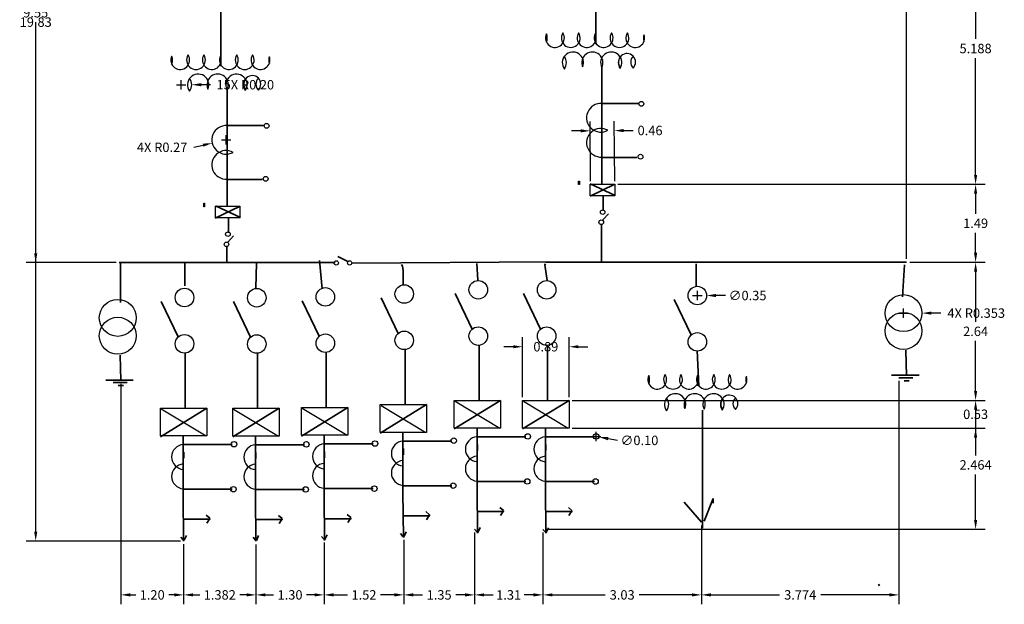
# Model space of a CAD drawing. Units: millimetres. Extents: x -4 to 31.8, y -11 to 11.2.
# Tile 1 of 2: x 13 to 31.8, y -11 to 0.1. Entities that reach past the tile are written whole.
import ezdxf

# ---------------------------------------------------------------- set-up
doc = ezdxf.new("R2010")
doc.units = ezdxf.units.MM
doc.header["$MEASUREMENT"] = 0
for name, color, linetype, lineweight in [('A-ANNO-DIMS', 2, 'Continuous', 18), ('E-ONEL-WIRE', 7, 'Continuous', 35), ('E-POWR-EQPM', 4, 'Continuous', 25)]:
    doc.layers.add(name, color=color, linetype=linetype, lineweight=lineweight)
doc.styles.get("Standard").update_dxf_attribs({"font": 'arial.ttf'})
doc.dimstyles.get("Standard").update_dxf_attribs({"dimtxt": 0.18, "dimasz": 0.18, "dimexe": 0.18, "dimexo": 0.0625, "dimgap": 0.09, "dimtad": 0, "dimtih": 1, "dimtoh": 1, "dimdec": 4, "dimzin": 0, "dimdsep": 46, "dimtxsty": 'Standard', "dimcen": 0.09, "dimadec": 0, "dimazin": 0, "dimtfac": 1, "dimtdec": 4, "dimtofl": 0, "dimtmove": 0, "dimatfit": 3, "dimfxl": 1, "dimtolj": 1, "dimtzin": 0, "dimarcsym": 0})

# ---------------------------------------------------------------- blocks, each defined once
blk = doc.blocks.new('XFMR-POWER')
for centre, radius, start, end in [((16.061, -0.651), 0.18, 154.6992, 32.9126), ((16.363, -0.651), 0.18, 147.0874, 32.9126), ((16.666, -0.651), 0.18, 147.0874, 25.3007), ((16.992, -0.651), 0.18, 154.6993, 32.9127), ((17.294, -0.651), 0.18, 147.0873, 32.9126), ((17.596, -0.651), 0.18, 147.0874, 20.5503), ((15.735, -0.651), 0.18, 334.6992, 25.3008), ((17.934, -0.651), 0.18, 159.4497, 200.5503), ((16.404, -1.122), 0.203, 336.2266, 216.7978), ((16.776, -1.122), 0.203, 332.4427, 203.7734), ((17.137, -1.122), 0.203, 326.0323, 207.5573), ((16.078, -1.122), 0.203, 323.2022, 36.7978), ((17.474, -1.122), 0.203, 146.0323, 213.9677), ((17.439, -1.11), 0.163, 315.5847, 221.0573), ((17.672, -1.11), 0.163, 135.5847, 224.4153)]:
    blk.add_arc(centre, radius, start, end)
blk = doc.blocks.new('CB-BREAKER')
blk.add_line((15.7, -7.316), (16.556, -7.832))
blk.add_lwpolyline([(15.685, -7.301), (16.571, -7.301), (16.571, -7.832), (15.685, -7.832)], close=True)
blk = doc.blocks.new('XFMR-AUX-LARGE')
for centre in [(14.868, -5.577), (14.868, -5.918)]:
    blk.add_circle(centre, 0.353)
blk = doc.blocks.new('*D7')
at = {"layer": 'A-ANNO-DIMS', "color": 0, "lineweight": -2, "transparency": 16777216}
for p, q in [((14.324, 5.091), (14.324, 11.195)), ((29.944, -4.451), (29.944, 11.195)), ((14.504, 11.015), (21.75, 11.015)), ((29.764, 11.015), (22.518, 11.015))]:
    blk.add_line(p, q, dxfattribs=at)
at = {"layer": 'A-ANNO-DIMS', "color": 0, "transparency": 16777216}
for points in [[(14.504, 11.045), (14.504, 10.985), (14.324, 11.015)], [(29.764, 11.045), (29.764, 10.985), (29.944, 11.015)]]:
    blk.add_solid(points, dxfattribs=at)
at = {"layer": 'Defpoints', "color": 0, "transparency": 16777216}
for p in [(29.944, 11.015), (14.324, 5.028), (29.944, -4.514)]:
    blk.add_point(p, dxfattribs=at)
at = {"layer": 'A-ANNO-DIMS', "color": 0, "transparency": 16777216, "insert": (22.134, 11.015), "char_height": 0.18, "attachment_point": 5}
blk.add_mtext('\\A1;15.62', dxfattribs=at)
blk = doc.blocks.new('*D13')
at = {"layer": 'A-ANNO-DIMS', "color": 0, "lineweight": -2, "transparency": 16777216}
for p, q in [((19.924, 9.99), (13.119, 9.99)), ((13.299, 9.81), (13.299, 0.256)), ((13.299, -9.661), (13.299, -0.108)), ((16.065, -9.841), (13.119, -9.841))]:
    blk.add_line(p, q, dxfattribs=at)
at = {"layer": 'A-ANNO-DIMS', "color": 0, "transparency": 16777216}
for points in [[(13.269, 9.81), (13.329, 9.81), (13.299, 9.99)], [(13.269, -9.661), (13.329, -9.661), (13.299, -9.841)]]:
    blk.add_solid(points, dxfattribs=at)
at = {"layer": 'Defpoints', "color": 0, "transparency": 16777216}
for p in [(13.299, 9.99), (19.987, 9.99), (16.127, -9.841)]:
    blk.add_point(p, dxfattribs=at)
at = {"layer": 'A-ANNO-DIMS', "color": 0, "transparency": 16777216, "insert": (13.299, 0.074), "char_height": 0.18, "attachment_point": 5}
blk.add_mtext('\\A1;19.83', dxfattribs=at)
blk = doc.blocks.new('*D14')
at = {"layer": 'A-ANNO-DIMS', "color": 0, "lineweight": -2, "transparency": 16777216}
for p, q in [((14.262, 5.028), (13.119, 5.028)), ((13.299, 4.848), (13.299, 0.435)), ((13.299, -4.342), (13.299, 0.071)), ((14.834, -4.522), (13.119, -4.522))]:
    blk.add_line(p, q, dxfattribs=at)
at = {"layer": 'A-ANNO-DIMS', "color": 0, "transparency": 16777216}
for points in [[(13.269, 4.848), (13.329, 4.848), (13.299, 5.028)], [(13.269, -4.342), (13.329, -4.342), (13.299, -4.522)]]:
    blk.add_solid(points, dxfattribs=at)
at = {"layer": 'Defpoints', "color": 0, "transparency": 16777216}
for p in [(13.299, 5.028), (14.324, 5.028), (14.897, -4.522)]:
    blk.add_point(p, dxfattribs=at)
at = {"layer": 'A-ANNO-DIMS', "color": 0, "transparency": 16777216, "insert": (13.299, 0.253), "char_height": 0.18, "attachment_point": 5}
blk.add_mtext('\\A1;9.55', dxfattribs=at)
blk = doc.blocks.new('*D18')
at = {"layer": 'A-ANNO-DIMS', "color": 0, "lineweight": -2, "transparency": 16777216}
for p, q in [((24.519, 2.164), (31.446, 2.164)), ((31.266, 1.984), (31.266, -0.248)), ((31.266, -2.844), (31.266, -0.612)), ((24.43, -3.024), (31.446, -3.024))]:
    blk.add_line(p, q, dxfattribs=at)
at = {"layer": 'A-ANNO-DIMS', "color": 0, "transparency": 16777216}
for points in [[(31.236, 1.984), (31.296, 1.984), (31.266, 2.164)], [(31.236, -2.844), (31.296, -2.844), (31.266, -3.024)]]:
    blk.add_solid(points, dxfattribs=at)
at = {"layer": 'Defpoints', "color": 0, "transparency": 16777216}
for p in [(24.456, 2.164), (31.266, 2.164), (24.367, -3.024)]:
    blk.add_point(p, dxfattribs=at)
at = {"layer": 'A-ANNO-DIMS', "color": 0, "transparency": 16777216, "insert": (31.266, -0.43), "char_height": 0.18, "attachment_point": 5}
blk.add_mtext('\\A1;5.188', dxfattribs=at)
blk = doc.blocks.new('*D19')
at = {"layer": 'A-ANNO-DIMS', "color": 0, "lineweight": -2, "transparency": 16777216}
for p, q in [((24.43, -3.024), (31.446, -3.024)), ((31.266, -3.204), (31.266, -3.587)), ((31.266, -4.334), (31.266, -3.951)), ((30.006, -4.514), (31.446, -4.514))]:
    blk.add_line(p, q, dxfattribs=at)
at = {"layer": 'A-ANNO-DIMS', "color": 0, "transparency": 16777216}
for points in [[(31.236, -3.204), (31.296, -3.204), (31.266, -3.024)], [(31.236, -4.334), (31.296, -4.334), (31.266, -4.514)]]:
    blk.add_solid(points, dxfattribs=at)
at = {"layer": 'Defpoints', "color": 0, "transparency": 16777216}
for p in [(24.367, -3.024), (31.266, -3.024), (29.944, -4.514)]:
    blk.add_point(p, dxfattribs=at)
at = {"layer": 'A-ANNO-DIMS', "color": 0, "transparency": 16777216, "insert": (31.266, -3.769), "char_height": 0.18, "attachment_point": 5}
blk.add_mtext('\\A1;1.49', dxfattribs=at)
blk = doc.blocks.new('*D20')
at = {"layer": 'A-ANNO-DIMS', "color": 0, "lineweight": -2, "transparency": 16777216}
for p, q in [((30.006, -4.514), (31.446, -4.514)), ((31.266, -4.694), (31.266, -5.652)), ((31.266, -6.974), (31.266, -6.016)), ((23.556, -7.154), (31.446, -7.154))]:
    blk.add_line(p, q, dxfattribs=at)
at = {"layer": 'A-ANNO-DIMS', "color": 0, "transparency": 16777216}
for points in [[(31.236, -4.694), (31.296, -4.694), (31.266, -4.514)], [(31.236, -6.974), (31.296, -6.974), (31.266, -7.154)]]:
    blk.add_solid(points, dxfattribs=at)
at = {"layer": 'Defpoints', "color": 0, "transparency": 16777216}
for p in [(29.944, -4.514), (31.266, -4.514), (23.494, -7.154)]:
    blk.add_point(p, dxfattribs=at)
at = {"layer": 'A-ANNO-DIMS', "color": 0, "transparency": 16777216, "insert": (31.266, -5.834), "char_height": 0.18, "attachment_point": 5}
blk.add_mtext('\\A1;2.64', dxfattribs=at)
blk = doc.blocks.new('*D21')
at = {"layer": 'A-ANNO-DIMS', "color": 0, "lineweight": -2, "transparency": 16777216}
for p, q in [((23.556, -7.154), (31.446, -7.154)), ((31.266, -7.334), (31.266, -8.204)), ((31.266, -9.437), (31.266, -8.567)), ((23.056, -9.617), (31.446, -9.617))]:
    blk.add_line(p, q, dxfattribs=at)
at = {"layer": 'A-ANNO-DIMS', "color": 0, "transparency": 16777216}
for points in [[(31.236, -7.334), (31.296, -7.334), (31.266, -7.154)], [(31.236, -9.437), (31.296, -9.437), (31.266, -9.617)]]:
    blk.add_solid(points, dxfattribs=at)
at = {"layer": 'Defpoints', "color": 0, "transparency": 16777216}
for p in [(23.494, -7.154), (31.266, -7.154), (22.994, -9.617)]:
    blk.add_point(p, dxfattribs=at)
at = {"layer": 'A-ANNO-DIMS', "color": 0, "transparency": 16777216, "insert": (31.266, -8.386), "char_height": 0.18, "attachment_point": 5}
blk.add_mtext('\\A1;2.464', dxfattribs=at)
blk = doc.blocks.new('*D22')
at = {"layer": 'A-ANNO-DIMS', "color": 0, "lineweight": -2, "transparency": 16777216}
for p, q in [((31.266, -6.974), (31.266, -6.794)), ((23.556, -7.154), (31.446, -7.154)), ((23.556, -7.685), (31.446, -7.685)), ((31.266, -7.865), (31.266, -8.045))]:
    blk.add_line(p, q, dxfattribs=at)
at = {"layer": 'A-ANNO-DIMS', "color": 0, "transparency": 16777216}
for points in [[(31.236, -6.974), (31.296, -6.974), (31.266, -7.154)], [(31.236, -7.865), (31.296, -7.865), (31.266, -7.685)]]:
    blk.add_solid(points, dxfattribs=at)
at = {"layer": 'Defpoints', "color": 0, "transparency": 16777216}
for p in [(23.494, -7.154), (23.494, -7.685), (31.266, -7.685)]:
    blk.add_point(p, dxfattribs=at)
at = {"layer": 'A-ANNO-DIMS', "color": 0, "transparency": 16777216, "insert": (31.266, -7.419), "char_height": 0.18, "attachment_point": 5}
blk.add_mtext('\\A1;0.53', dxfattribs=at)
blk = doc.blocks.new('*D23')
at = {"layer": 'A-ANNO-DIMS', "color": 0, "lineweight": -2, "transparency": 16777216}
for p, q in [((14.925612, -6.837922), (14.925612, -11.049806)), ((16.127036, -9.903339), (16.127036, -11.049806)), ((15.105612, -10.869806), (15.211324, -10.869806)), ((15.947036, -10.869806), (15.841324, -10.869806))]:
    blk.add_line(p, q, dxfattribs=at)
at = {"layer": 'A-ANNO-DIMS', "color": 0, "transparency": 16777216}
for points in [[(15.105612, -10.839806), (15.105612, -10.899806), (14.925612, -10.869806)], [(15.947036, -10.839806), (15.947036, -10.899806), (16.127036, -10.869806)]]:
    blk.add_solid(points, dxfattribs=at)
at = {"layer": 'Defpoints', "color": 0, "transparency": 16777216}
for p in [(14.925612, -6.775422), (16.127036, -9.840839), (16.127036, -10.869806)]:
    blk.add_point(p, dxfattribs=at)
at = {"layer": 'A-ANNO-DIMS', "color": 0, "transparency": 16777216, "insert": (15.526324, -10.869806), "char_height": 0.18, "attachment_point": 5}
blk.add_mtext('\\A1;1.20', dxfattribs=at)
blk = doc.blocks.new('*D24')
at = {"layer": 'A-ANNO-DIMS', "color": 0, "lineweight": -2, "transparency": 16777216}
for p, q in [((16.127, -9.903), (16.127, -11.05)), ((17.509, -9.907), (17.509, -11.05)), ((16.307, -10.87), (16.434, -10.87)), ((17.329, -10.87), (17.202, -10.87))]:
    blk.add_line(p, q, dxfattribs=at)
at = {"layer": 'A-ANNO-DIMS', "color": 0, "transparency": 16777216}
for points in [[(16.307, -10.84), (16.307, -10.9), (16.127, -10.87)], [(17.329, -10.84), (17.329, -10.9), (17.509, -10.87)]]:
    blk.add_solid(points, dxfattribs=at)
at = {"layer": 'Defpoints', "color": 0, "transparency": 16777216}
for p in [(16.127, -9.841), (17.509, -9.845), (17.509, -10.87)]:
    blk.add_point(p, dxfattribs=at)
at = {"layer": 'A-ANNO-DIMS', "color": 0, "transparency": 16777216, "insert": (16.818, -10.87), "char_height": 0.18, "attachment_point": 5}
blk.add_mtext('\\A1;1.382', dxfattribs=at)
blk = doc.blocks.new('*D25')
at = {"layer": 'A-ANNO-DIMS', "color": 0, "lineweight": -2, "transparency": 16777216}
for p, q in [((17.509, -9.907), (17.509, -11.05)), ((18.813, -9.872), (18.813, -11.05)), ((17.689, -10.87), (17.846, -10.87)), ((18.633, -10.87), (18.476, -10.87))]:
    blk.add_line(p, q, dxfattribs=at)
at = {"layer": 'A-ANNO-DIMS', "color": 0, "transparency": 16777216}
for points in [[(17.689, -10.84), (17.689, -10.9), (17.509, -10.87)], [(18.633, -10.84), (18.633, -10.9), (18.813, -10.87)]]:
    blk.add_solid(points, dxfattribs=at)
at = {"layer": 'Defpoints', "color": 0, "transparency": 16777216}
for p in [(17.509, -9.845), (18.813, -9.809), (18.813, -10.87)]:
    blk.add_point(p, dxfattribs=at)
at = {"layer": 'A-ANNO-DIMS', "color": 0, "transparency": 16777216, "insert": (18.161, -10.87), "char_height": 0.18, "attachment_point": 5}
blk.add_mtext('\\A1;1.30', dxfattribs=at)
blk = doc.blocks.new('*D26')
at = {"layer": 'A-ANNO-DIMS', "color": 0, "lineweight": -2, "transparency": 16777216}
for p, q in [((18.813, -9.872), (18.813, -11.05)), ((20.336, -9.821), (20.336, -11.05)), ((18.993, -10.87), (19.26, -10.87)), ((20.156, -10.87), (19.889, -10.87))]:
    blk.add_line(p, q, dxfattribs=at)
at = {"layer": 'A-ANNO-DIMS', "color": 0, "transparency": 16777216}
for points in [[(18.993, -10.84), (18.993, -10.9), (18.813, -10.87)], [(20.156, -10.84), (20.156, -10.9), (20.336, -10.87)]]:
    blk.add_solid(points, dxfattribs=at)
at = {"layer": 'Defpoints', "color": 0, "transparency": 16777216}
for p in [(20.336, -9.758), (18.813, -9.809), (20.336, -10.87)]:
    blk.add_point(p, dxfattribs=at)
at = {"layer": 'A-ANNO-DIMS', "color": 0, "transparency": 16777216, "insert": (19.574, -10.87), "char_height": 0.18, "attachment_point": 5}
blk.add_mtext('\\A1;1.52', dxfattribs=at)
blk = doc.blocks.new('*D27')
at = {"layer": 'A-ANNO-DIMS', "color": 0, "lineweight": -2, "transparency": 16777216}
for p, q in [((21.687, -9.679), (21.687, -11.05)), ((20.336, -9.821), (20.336, -11.05)), ((20.516, -10.87), (20.695, -10.87)), ((21.507, -10.87), (21.327, -10.87))]:
    blk.add_line(p, q, dxfattribs=at)
at = {"layer": 'A-ANNO-DIMS', "color": 0, "transparency": 16777216}
for points in [[(20.516, -10.84), (20.516, -10.9), (20.336, -10.87)], [(21.507, -10.84), (21.507, -10.9), (21.687, -10.87)]]:
    blk.add_solid(points, dxfattribs=at)
at = {"layer": 'Defpoints', "color": 0, "transparency": 16777216}
for p in [(20.336, -9.758), (21.687, -9.617), (21.687, -10.87)]:
    blk.add_point(p, dxfattribs=at)
at = {"layer": 'A-ANNO-DIMS', "color": 0, "transparency": 16777216, "insert": (21.011, -10.87), "char_height": 0.18, "attachment_point": 5}
blk.add_mtext('\\A1;1.35', dxfattribs=at)
blk = doc.blocks.new('*D28')
at = {"layer": 'A-ANNO-DIMS', "color": 0, "lineweight": -2, "transparency": 16777216}
for p, q in [((21.687, -9.679), (21.687, -11.05)), ((22.994, -9.68), (22.994, -11.05)), ((21.867, -10.87), (22.042, -10.87)), ((22.814, -10.87), (22.638, -10.87))]:
    blk.add_line(p, q, dxfattribs=at)
at = {"layer": 'A-ANNO-DIMS', "color": 0, "transparency": 16777216}
for points in [[(21.867, -10.84), (21.867, -10.9), (21.687, -10.87)], [(22.814, -10.84), (22.814, -10.9), (22.994, -10.87)]]:
    blk.add_solid(points, dxfattribs=at)
at = {"layer": 'Defpoints', "color": 0, "transparency": 16777216}
for p in [(21.687, -9.617), (22.994, -9.617), (22.994, -10.87)]:
    blk.add_point(p, dxfattribs=at)
at = {"layer": 'A-ANNO-DIMS', "color": 0, "transparency": 16777216, "insert": (22.34, -10.87), "char_height": 0.18, "attachment_point": 5}
blk.add_mtext('\\A1;1.31', dxfattribs=at)
blk = doc.blocks.new('*D29')
at = {"layer": 'A-ANNO-DIMS', "color": 0, "lineweight": -2, "transparency": 16777216}
for p, q in [((26.026, -9.543), (26.026, -11.05)), ((22.994, -9.68), (22.994, -11.05)), ((23.174, -10.87), (24.186, -10.87)), ((25.846, -10.87), (24.833, -10.87))]:
    blk.add_line(p, q, dxfattribs=at)
at = {"layer": 'A-ANNO-DIMS', "color": 0, "transparency": 16777216}
for points in [[(23.174, -10.84), (23.174, -10.9), (22.994, -10.87)], [(25.846, -10.84), (25.846, -10.9), (26.026, -10.87)]]:
    blk.add_solid(points, dxfattribs=at)
at = {"layer": 'Defpoints', "color": 0, "transparency": 16777216}
for p in [(26.026, -9.48), (22.994, -9.617), (26.026, -10.87)]:
    blk.add_point(p, dxfattribs=at)
at = {"layer": 'A-ANNO-DIMS', "color": 0, "transparency": 16777216, "insert": (24.51, -10.87), "char_height": 0.18, "attachment_point": 5}
blk.add_mtext('\\A1;3.03', dxfattribs=at)
blk = doc.blocks.new('*D30')
at = {"layer": 'A-ANNO-DIMS', "color": 0, "lineweight": -2, "transparency": 16777216}
for p, q in [((29.8, -6.783), (29.8, -11.05)), ((26.026, -9.543), (26.026, -11.05)), ((26.206, -10.87), (27.52, -10.87)), ((29.62, -10.87), (28.306, -10.87))]:
    blk.add_line(p, q, dxfattribs=at)
at = {"layer": 'A-ANNO-DIMS', "color": 0, "transparency": 16777216}
for points in [[(26.206, -10.84), (26.206, -10.9), (26.026, -10.87)], [(29.62, -10.84), (29.62, -10.9), (29.8, -10.87)]]:
    blk.add_solid(points, dxfattribs=at)
at = {"layer": 'Defpoints', "color": 0, "transparency": 16777216}
for p in [(29.8, -6.72), (26.026, -9.48), (29.8, -10.87)]:
    blk.add_point(p, dxfattribs=at)
at = {"layer": 'A-ANNO-DIMS', "color": 0, "transparency": 16777216, "insert": (27.913, -10.87), "char_height": 0.18, "attachment_point": 5}
blk.add_mtext('\\A1;3.774', dxfattribs=at)
blk = doc.blocks.new('*D31')
at = {"layer": 'A-ANNO-DIMS', "color": 0, "lineweight": -2, "transparency": 16777216}
for p, q in [((22.607382, -7.091185), (22.607382, -5.948685)), ((23.4935, -7.091185), (23.4935, -5.948685)), ((22.427382, -6.128685), (22.247382, -6.128685)), ((23.6735, -6.128685), (23.8535, -6.128685))]:
    blk.add_line(p, q, dxfattribs=at)
at = {"layer": 'A-ANNO-DIMS', "color": 0, "transparency": 16777216}
for points in [[(22.427382, -6.098685), (22.427382, -6.158685), (22.607382, -6.128685)], [(23.6735, -6.098685), (23.6735, -6.158685), (23.4935, -6.128685)]]:
    blk.add_solid(points, dxfattribs=at)
at = {"layer": 'Defpoints', "color": 0, "transparency": 16777216}
for p in [(23.4935, -6.128685), (22.607382, -7.153685), (23.4935, -7.153685)]:
    blk.add_point(p, dxfattribs=at)
at = {"layer": 'A-ANNO-DIMS', "color": 0, "transparency": 16777216, "insert": (23.050441, -6.128685), "char_height": 0.18, "attachment_point": 5}
blk.add_mtext('\\A1;0.89', dxfattribs=at)
blk = doc.blocks.new('*D33')
at = {"layer": 'A-ANNO-DIMS', "color": 0, "lineweight": -2, "transparency": 16777216}
for p, q in [((23.907, -2.965), (23.898, -1.823)), ((24.367, -2.962), (24.358, -1.819)), ((23.719, -2.004), (23.539, -2.006)), ((24.539, -1.998), (24.719, -1.996))]:
    blk.add_line(p, q, dxfattribs=at)
at = {"layer": 'A-ANNO-DIMS', "color": 0, "transparency": 16777216}
for points in [[(23.719, -1.974), (23.719, -2.034), (23.899, -2.003)], [(24.539, -1.968), (24.539, -2.028), (24.359, -1.999)]]:
    blk.add_solid(points, dxfattribs=at)
at = {"layer": 'Defpoints', "color": 0, "transparency": 16777216}
for p in [(24.359, -1.999), (23.907, -3.028), (24.367, -3.024)]:
    blk.add_point(p, dxfattribs=at)
at = {"layer": 'A-ANNO-DIMS', "color": 0, "transparency": 16777216, "insert": (25.043, -1.996), "char_height": 0.18, "attachment_point": 5}
blk.add_mtext('\\A1;0.46', dxfattribs=at)
blk = doc.blocks.new('*D34')
at = {"layer": 'A-ANNO-DIMS', "color": 0, "lineweight": -2, "transparency": 16777216}
for p, q in [((29.888, -5.576), (29.888, -5.396)), ((29.798, -5.486), (29.978, -5.486)), ((30.601, -5.486), (30.421, -5.486))]:
    blk.add_line(p, q, dxfattribs=at)
at = {"layer": 'A-ANNO-DIMS', "color": 0, "transparency": 16777216}
blk.add_solid([(30.421, -5.456), (30.421, -5.516), (30.241, -5.486)], dxfattribs=at)
at = {"layer": 'Defpoints', "color": 0, "transparency": 16777216}
for p in [(29.888, -5.486), (30.241, -5.486)]:
    blk.add_point(p, dxfattribs=at)
at = {"layer": 'A-ANNO-DIMS', "color": 0, "transparency": 16777216, "insert": (31.278, -5.486), "char_height": 0.18, "attachment_point": 5}
blk.add_mtext('\\A1;4X R0.353', dxfattribs=at)
blk = doc.blocks.new('*D36')
at = {"layer": 'A-ANNO-DIMS', "color": 0, "lineweight": -2, "transparency": 16777216}
for p, q in [((16.849, -2.176), (17.029, -2.176)), ((16.939, -2.266), (16.939, -2.086)), ((16.322, -2.318), (16.497, -2.277))]:
    blk.add_line(p, q, dxfattribs=at)
at = {"layer": 'A-ANNO-DIMS', "color": 0, "transparency": 16777216}
blk.add_solid([(16.491, -2.248), (16.504, -2.307), (16.673, -2.237)], dxfattribs=at)
at = {"layer": 'Defpoints', "color": 0, "transparency": 16777216}
for p in [(16.673, -2.237), (16.939, -2.176)]:
    blk.add_point(p, dxfattribs=at)
at = {"layer": 'A-ANNO-DIMS', "color": 0, "transparency": 16777216, "insert": (15.715, -2.318), "char_height": 0.18, "attachment_point": 5}
blk.add_mtext('\\A1;4X R0.27', dxfattribs=at)
blk = doc.blocks.new('*D39')
at = {"layer": 'A-ANNO-DIMS', "color": 0, "lineweight": -2, "transparency": 16777216}
for p, q in [((15.988, -1.122), (16.168, -1.122)), ((16.078, -1.212), (16.078, -1.032)), ((16.642, -1.122), (16.462, -1.122))]:
    blk.add_line(p, q, dxfattribs=at)
at = {"layer": 'A-ANNO-DIMS', "color": 0, "transparency": 16777216}
blk.add_solid([(16.462, -1.092), (16.462, -1.152), (16.282, -1.122)], dxfattribs=at)
at = {"layer": 'Defpoints', "color": 0, "transparency": 16777216}
for p in [(16.078, -1.122), (16.282, -1.122)]:
    blk.add_point(p, dxfattribs=at)
at = {"layer": 'A-ANNO-DIMS', "color": 0, "transparency": 16777216, "insert": (17.306, -1.122), "char_height": 0.18, "attachment_point": 5}
blk.add_mtext('\\A1;15X R0.20', dxfattribs=at)
blk = doc.blocks.new('*D40')
at = {"layer": 'A-ANNO-DIMS', "color": 0, "lineweight": -2, "transparency": 16777216}
for p, q in [((25.947, -5.24), (25.947, -5.06)), ((25.857, -5.15), (26.037, -5.15)), ((26.484, -5.15), (26.304, -5.15))]:
    blk.add_line(p, q, dxfattribs=at)
at = {"layer": 'A-ANNO-DIMS', "color": 0, "transparency": 16777216}
blk.add_solid([(26.304, -5.12), (26.304, -5.18), (26.124, -5.15)], dxfattribs=at)
at = {"layer": 'Defpoints', "color": 0, "transparency": 16777216}
for p in [(25.77, -5.15), (26.124, -5.15)]:
    blk.add_point(p, dxfattribs=at)
at = {"layer": 'A-ANNO-DIMS', "color": 0, "transparency": 16777216, "insert": (26.907, -5.15), "char_height": 0.18, "attachment_point": 5}
blk.add_mtext('\\A1;∅0.35', dxfattribs=at)
blk = doc.blocks.new('*D42')
at = {"layer": 'A-ANNO-DIMS', "color": 0, "lineweight": -2, "transparency": 16777216}
for p, q in [((23.923, -7.843), (24.103, -7.843)), ((24.013, -7.933), (24.013, -7.753)), ((24.418, -7.918), (24.241, -7.885))]:
    blk.add_line(p, q, dxfattribs=at)
at = {"layer": 'A-ANNO-DIMS', "color": 0, "transparency": 16777216}
blk.add_solid([(24.247, -7.856), (24.236, -7.915), (24.064, -7.853)], dxfattribs=at)
at = {"layer": 'Defpoints', "color": 0, "transparency": 16777216}
for p in [(23.961, -7.834), (24.064, -7.853)]:
    blk.add_point(p, dxfattribs=at)
at = {"layer": 'A-ANNO-DIMS', "color": 0, "transparency": 16777216, "insert": (24.84, -7.918), "char_height": 0.18, "attachment_point": 5}
blk.add_mtext('\\A1;∅0.10', dxfattribs=at)

msp = doc.modelspace()

# ---------------------------------------------------------------- linework, layer by layer
at = {"layer": 'E-ONEL-WIRE'}
for p, q in [((16.8405, 1.2045), (16.8405, 0.0598)), ((24.0041, 0.5211), (24.0041, -0.2518)), ((16.8404, 0.0996), (16.8404, -0.6732)), ((16.8405, 0.0598), (16.8405, 0.0772)), ((24.0041, -0.2518), (24.0041, -0.3447)), ((16.8404, -0.6732), (16.8404, -0.7662)), ((24.1204, -0.7644), (24.1204, -1.6128)), ((16.9567, -1.1858), (16.9567, -2.0342)), ((24.1203, -1.4814), (24.8299, -1.4814)), ((24.1204, -1.6128), (24.1204, -1.8801)), ((24.1204, -1.8801), (24.1204, -3.0155)), ((16.9566, -1.9029), (17.6662, -1.9029)), ((16.9567, -2.0342), (16.9567, -2.3015)), ((16.9567, -2.3015), (16.9567, -3.437)), ((24.1319, -2.51), (24.7892, -2.51)), ((16.9682, -2.9314), (17.6255, -2.9314)), ((24.3599, -3.0277), (23.8963, -3.2502)), ((23.8999, -3.0168), (24.3745, -3.2393)), ((24.1481, -3.2393), (24.1481, -3.531)), ((17.1961, -3.4492), (16.7326, -3.6717)), ((16.7362, -3.4383), (17.2107, -3.6607)), ((16.9844, -3.6607), (16.9844, -3.9525)), ((24.1372, -3.706), (24.2467, -3.5893)), ((24.1141, -3.792), (24.1141, -4.5047)), ((16.9735, -4.1275), (17.083, -4.0108)), ((16.9552, -4.2193), (16.9552, -4.4636)), ((14.9215, -4.512), (14.9215, -5.2827)), ((16.9552, -4.4636), (16.9552, -4.5293)), ((18.7743, -5.023), (18.7221, -4.4808)), ((19.2667, -4.4979), (19.0769, -4.4067)), ((19.3434, -4.5307), (23.0958, -4.5088)), ((23.0493, -4.5139), (29.9436, -4.5139)), ((19.0247, -4.522), (14.8965, -4.522)), ((16.1467, -4.5319), (16.1467, -4.9617)), ((17.5097, -5.0055), (17.5201, -4.5297)), ((20.3132, -4.5893), (20.2922, -4.5579)), ((20.3237, -4.6731), (20.3132, -4.5893)), ((20.3237, -4.9558), (20.3237, -4.6731)), ((21.7503, -4.8563), (21.7292, -4.5396)), ((23.0318, -4.5628), (23.0424, -4.5416)), ((23.0742, -4.8597), (23.0318, -4.5628)), ((25.9216, -4.9785), (25.9216, -4.5439)), ((29.9049, -4.5617), (29.8697, -5.1776)), ((16.0249, -5.9406), (15.7, -5.2619)), ((17.407, -5.9446), (17.0821, -5.2658)), ((18.7185, -5.929), (18.3936, -5.2503)), ((20.2259, -5.8739), (19.901, -5.1952)), ((21.6407, -5.7922), (21.3158, -5.1135)), ((22.9474, -5.793), (22.6225, -5.1143)), ((25.829, -5.9028), (25.5041, -5.224)), ((20.3585, -6.1722), (20.3585, -7.2345)), ((21.7733, -6.0905), (21.7733, -7.1529)), ((23.08, -6.0913), (23.08, -7.1537)), ((25.9418, -6.1982), (25.977, -6.8845)), ((29.9314, -6.1963), (29.9451, -6.6844)), ((14.9119, -6.2874), (14.9256, -6.7754)), ((16.1575, -6.2389), (16.1575, -7.3012)), ((17.5396, -6.2428), (17.5396, -7.3052)), ((18.8511, -6.2273), (18.8511, -7.2896)), ((14.6367, -6.7658), (15.1648, -6.7658)), ((29.6563, -6.6747), (30.1843, -6.6747)), ((29.7997, -6.7203), (30.0669, -6.7203)), ((14.7802, -6.8114), (15.0474, -6.8114)), ((14.8779, -6.87), (14.9757, -6.87)), ((21.7733, -6.9906), (21.7733, -6.9316)), ((23.08, -6.9914), (23.08, -6.9324)), ((25.9591, -6.7797), (25.9591, -6.8727)), ((29.8975, -6.7789), (29.9952, -6.7789)), ((16.1575, -7.1389), (16.1575, -7.0799)), ((17.5396, -7.1429), (17.5396, -7.0839)), ((18.8511, -7.1273), (18.8511, -7.0683)), ((20.3585, -7.0722), (20.3585, -7.0132)), ((16.5711, -7.3012), (15.6849, -7.8471)), ((17.9531, -7.3052), (17.067, -7.8511)), ((19.2646, -7.2896), (18.3785, -7.8355)), ((20.772, -7.2345), (19.8859, -7.7804)), ((22.1868, -7.1529), (21.3007, -7.6988)), ((23.4935, -7.1537), (22.6074, -7.6996)), ((26.0434, -7.3425), (26.0434, -9.5848)), ((21.7347, -7.6912), (21.7347, -8.836)), ((23.0414, -7.692), (23.0414, -8.8368)), ((16.1189, -7.8396), (16.1189, -8.9843)), ((17.5009, -7.8435), (17.5009, -8.9883)), ((18.8125, -7.8279), (18.8125, -8.9727)), ((20.3199, -7.7728), (20.3199, -8.9176)), ((21.7405, -7.8481), (22.6711, -7.8481)), ((23.0472, -7.8489), (23.9778, -7.8489)), ((16.1247, -7.9964), (17.0554, -7.9964)), ((17.5068, -8.0004), (18.4374, -8.0004)), ((18.8183, -7.9848), (19.749, -7.9848)), ((20.3257, -7.9297), (21.2564, -7.9297)), ((20.329, -8.1936), (20.329, -8.0755)), ((20.329, -8.0755), (20.329, -8.0755)), ((21.7437, -8.1119), (21.7437, -7.9939)), ((21.7437, -7.9939), (21.7437, -7.9939)), ((23.0504, -8.1127), (23.0504, -7.9947)), ((23.0504, -7.9947), (23.0504, -7.9947)), ((16.128, -8.2603), (16.128, -8.1422)), ((16.128, -8.1422), (16.128, -8.1422)), ((17.51, -8.2642), (17.51, -8.1462)), ((17.51, -8.1462), (17.51, -8.1462)), ((18.8216, -8.2487), (18.8216, -8.1306)), ((18.8216, -8.1306), (18.8216, -8.1306)), ((18.8183, -8.8391), (19.749, -8.8391)), ((20.3257, -8.784), (21.2564, -8.784)), ((21.7428, -9.6925), (21.7347, -8.8185)), ((21.7405, -8.7023), (22.6711, -8.7023)), ((23.0495, -9.6933), (23.0414, -8.8193)), ((23.0472, -8.7031), (23.9778, -8.7031)), ((16.127, -9.8408), (16.1189, -8.9669)), ((16.1247, -8.8507), (17.0554, -8.8507)), ((17.5091, -9.8448), (17.5009, -8.9709)), ((17.5068, -8.8546), (18.4374, -8.8546)), ((18.8206, -9.8292), (18.8125, -8.9553)), ((20.328, -9.7741), (20.3199, -8.9002)), ((26.0782, -9.4631), (26.2522, -9.0285)), ((26.2522, -9.0285), (26.2522, -9.1155)), ((22.2421, -9.2575), (22.1742, -9.1976)), ((23.5488, -9.2583), (23.4809, -9.1984)), ((26.026, -9.4805), (25.6954, -9.0981)), ((16.6264, -9.4058), (16.5584, -9.346)), ((16.6264, -9.4098), (16.5704, -9.5016)), ((16.6264, -9.4098), (16.6264, -9.4258)), ((18.0084, -9.4098), (17.9405, -9.35)), ((19.3199, -9.3942), (19.252, -9.3344)), ((19.3199, -9.3982), (19.264, -9.49)), ((19.3199, -9.3982), (19.3199, -9.4142)), ((20.3287, -9.3586), (20.8358, -9.3586)), ((20.8273, -9.3391), (20.7594, -9.2793)), ((20.8273, -9.3431), (20.7714, -9.4349)), ((20.8273, -9.3431), (20.8273, -9.3591)), ((21.7434, -9.277), (22.2506, -9.277)), ((22.2421, -9.2615), (22.1862, -9.3533)), ((22.2421, -9.2615), (22.2421, -9.2775)), ((23.0501, -9.2778), (23.5573, -9.2778)), ((23.5488, -9.2623), (23.4929, -9.3541)), ((23.5488, -9.2623), (23.5488, -9.2783)), ((16.1277, -9.4253), (16.6348, -9.4253)), ((17.5097, -9.4293), (18.0169, -9.4293)), ((18.0084, -9.4138), (17.9524, -9.5056)), ((18.0084, -9.4138), (18.0084, -9.4298)), ((18.8213, -9.4137), (19.3284, -9.4137)), ((21.7508, -9.6765), (21.7947, -9.5847)), ((23.0575, -9.6773), (23.1014, -9.5856)), ((26.0434, -9.5848), (26.0608, -9.5848)), ((16.119, -9.8209), (16.0711, -9.765)), ((16.135, -9.8249), (16.179, -9.7331)), ((17.5011, -9.8249), (17.4531, -9.769)), ((17.517, -9.8288), (17.561, -9.7371)), ((18.8126, -9.8093), (18.7647, -9.7534)), ((18.8286, -9.8133), (18.8725, -9.7215)), ((20.32, -9.7542), (20.2721, -9.6983)), ((20.336, -9.7582), (20.3799, -9.6664)), ((21.7348, -9.6725), (21.6868, -9.6167)), ((23.0415, -9.6733), (22.9935, -9.6175)), ((29.4319, -10.6958), (29.4109, -10.6644))]:
    msp.add_line(p, q, dxfattribs=at)
at = {"layer": 'E-POWR-EQPM'}
for points in [[(23.6919, -3.0314), (23.6736, -3.0314), (23.6736, -2.9621), (23.6919, -2.9621)], [(23.6919, -2.973), (23.6773, -2.973), (23.6773, -2.9876), (23.6919, -2.9876)], [(23.8999, -3.0241), (24.3672, -3.0241), (24.3672, -3.2466), (23.8999, -3.2466)], [(23.9072, -3.0277), (23.9875, -3.0277), (23.9875, -3.0277), (23.9072, -3.0277)], [(16.5282, -3.4528), (16.5099, -3.4528), (16.5099, -3.3836), (16.5282, -3.3836)], [(16.5282, -3.3945), (16.5136, -3.3945), (16.5136, -3.4091), (16.5282, -3.4091)], [(16.7362, -3.4456), (17.2034, -3.4456), (17.2034, -3.668), (16.7362, -3.668)], [(16.7435, -3.4492), (16.8238, -3.4492), (16.8238, -3.4492), (16.7435, -3.4492)]]:
    msp.add_lwpolyline(points, close=True, dxfattribs=at)
for centre, radius in [((24.8764, -1.4872), 0.0465), ((17.7127, -1.9087), 0.0465), ((24.859, -2.4983), 0.0465), ((17.6953, -2.9198), 0.0465), ((24.1372, -3.5565), 0.044), ((24.1095, -3.7505), 0.044), ((16.9735, -3.978), 0.044), ((16.9458, -4.172), 0.044), ((19.0441, -4.527), 0.0402), ((19.055, -4.4906), 0.00365), ((19.2996, -4.527), 0.0402), ((21.7588, -5.0398), 0.1771), ((23.0655, -5.0406), 0.1771), ((16.1431, -5.1881), 0.1771), ((17.5251, -5.1921), 0.1771), ((18.8367, -5.1765), 0.1771), ((20.3441, -5.1214), 0.1771), ((25.9471, -5.1503), 0.1771), ((20.3441, -6.0067), 0.1771), ((21.7588, -5.925), 0.1771), ((23.0655, -5.9258), 0.1771), ((16.1431, -6.0734), 0.1771), ((17.5251, -6.0773), 0.1771), ((18.8367, -6.0618), 0.1771), ((25.9471, -6.0356), 0.1771), ((21.2913, -7.9239), 0.0523), ((22.706, -7.8423), 0.0523), ((24.0127, -7.8431), 0.0523), ((17.0903, -7.9906), 0.0523), ((18.4723, -7.9946), 0.0523), ((19.7838, -7.979), 0.0523), ((22.6944, -8.7023), 0.0523), ((24.0011, -8.7031), 0.0523), ((17.0786, -8.8507), 0.0523), ((18.4607, -8.8546), 0.0523), ((19.7722, -8.8391), 0.0523), ((21.2796, -8.784), 0.0523)]:
    msp.add_circle(centre, radius, dxfattribs=at)
for centre, radius, start, end in [((24.1028, -1.7545), 0.2734, 86.31794, 299.36433), ((16.9391, -2.176), 0.2734, 86.31794, 299.36433), ((24.1028, -2.231), 0.2734, 60.63567, 273.68206), ((16.9391, -2.6525), 0.2734, 60.63567, 273.68206), ((21.7521, -8.0864), 0.2385, 94.19612, 265.80388), ((23.0588, -8.0872), 0.2385, 94.19612, 265.80388), ((16.1364, -8.2347), 0.2385, 94.19612, 265.80388), ((17.5184, -8.2387), 0.2385, 94.19612, 265.80388), ((18.8299, -8.2231), 0.2385, 94.19612, 265.80388), ((20.3374, -8.168), 0.2385, 94.19612, 265.80388), ((21.7521, -8.4583), 0.2385, 94.19612, 265.80388), ((23.0588, -8.4591), 0.2385, 94.19612, 265.80388), ((16.1364, -8.6066), 0.2385, 94.19612, 265.80388), ((17.5184, -8.6106), 0.2385, 94.19612, 265.80388), ((18.8299, -8.595), 0.2385, 94.19612, 265.80388), ((20.3374, -8.5399), 0.2385, 94.19612, 265.80388)]:
    msp.add_arc(centre, radius, start, end, dxfattribs=at)

# ---------------------------------------------------------------- block references
for name, p in [('XFMR-POWER', (7.1637, 0.4215)), ('XFMR-POWER', (0, 0)), ('XFMR-AUX-LARGE', (0, 0)), ('XFMR-AUX-LARGE', (15.0195, 0.091)), ('XFMR-POWER', (9.1187, -6.1065)), ('CB-BREAKER', (0, 0)), ('CB-BREAKER', (1.382, -0.004)), ('CB-BREAKER', (2.6936, 0.0116)), ('CB-BREAKER', (4.201, 0.0667)), ('CB-BREAKER', (5.6157, 0.1483)), ('CB-BREAKER', (6.9224, 0.1475))]:
    msp.add_blockref(name, p, dxfattribs=at)

# ---------------------------------------------------------------- dimensions: what is measured, and where the dimension line sits
at = {"layer": 'A-ANNO-DIMS'}
for base, p1, p2, override, picture, middle in [((29.9436, 11.0146), (14.3245, 5.0281), (29.9436, -4.5139), {"dimdec": 2, "dimlfac": 1, "dimrnd": 0, "dimzin": 0, "dimdsep": 46, "dimlunit": 2}, '*D7', (22.134, 11.0146)), ((23.4935, -6.1287), (22.6074, -7.1537), (23.4935, -7.1537), {"dimdec": 2, "dimlfac": 1, "dimrnd": 0, "dimzin": 0, "dimdsep": 46, "dimlunit": 2}, '*D31', (23.0504, -6.1287)), ((16.127, -10.8698), (14.9256, -6.7754), (16.127, -9.8408), {"dimdec": 2, "dimlfac": 1, "dimrnd": 0, "dimzin": 0, "dimdsep": 46, "dimlunit": 2}, '*D23', (15.5263, -10.8698)), ((29.7997, -10.8698), (26.026, -9.4805), (29.7997, -6.7203), {"dimdec": 3, "dimlfac": 1, "dimrnd": 0, "dimzin": 0, "dimdsep": 46, "dimlunit": 2}, '*D30', (27.9128, -10.8698)), ((26.026, -10.8698), (22.9935, -9.6175), (26.026, -9.4805), {"dimdec": 2, "dimlfac": 1, "dimrnd": 0, "dimzin": 0, "dimdsep": 46, "dimlunit": 2}, '*D29', (24.5098, -10.8698)), ((20.336, -10.8698), (18.8126, -9.8093), (20.336, -9.7582), {"dimdec": 2, "dimlfac": 1, "dimrnd": 0, "dimzin": 0, "dimdsep": 46, "dimlunit": 2}, '*D26', (19.5743, -10.8698)), ((21.6868, -10.8698), (20.336, -9.7582), (21.6868, -9.6167), {"dimdec": 2, "dimlfac": 1, "dimrnd": 0, "dimzin": 0, "dimdsep": 46, "dimlunit": 2}, '*D27', (21.0114, -10.8698)), ((22.9935, -10.8698), (21.6868, -9.6167), (22.9935, -9.6175), {"dimdec": 2, "dimlfac": 1, "dimrnd": 0, "dimzin": 0, "dimdsep": 46, "dimlunit": 2}, '*D28', (22.3402, -10.8698)), ((17.5091, -10.8698), (16.127, -9.8408), (17.5091, -9.8448), {"dimdec": 3, "dimlfac": 1, "dimrnd": 0, "dimzin": 0, "dimdsep": 46, "dimlunit": 2}, '*D24', (16.818, -10.8698)), ((18.8126, -10.8698), (17.5091, -9.8448), (18.8126, -9.8093), {"dimdec": 2, "dimlfac": 1, "dimrnd": 0, "dimzin": 0, "dimdsep": 46, "dimlunit": 2}, '*D25', (18.1608, -10.8698))]:
    dim = msp.add_linear_dim(base=base, p1=p1, p2=p2, dimstyle='Standard', override=override, dxfattribs=at)
    dim.commit()
    dim.dimension.update_dxf_attribs({"geometry": picture, "text_midpoint": middle})
for base, p1, p2, angle, override, picture, middle in [((13.2995, 9.9896), (16.127, -9.8408), (19.9867, 9.9896), 90, {"dimdec": 2, "dimlfac": 1, "dimrnd": 0, "dimzin": 0, "dimdsep": 46, "dimlunit": 2}, '*D13', (13.2995, 0.0744)), ((13.2995, 5.0281), (14.8965, -4.522), (14.3245, 5.0281), 90, {"dimdec": 2, "dimlfac": 1, "dimrnd": 0, "dimzin": 0, "dimdsep": 46, "dimlunit": 2}, '*D14', (13.2995, 0.2531)), ((31.2659, 2.1643), (24.3672, -3.0241), (24.4564, 2.1643), 90, {"dimdec": 3, "dimlfac": 1, "dimrnd": 0, "dimzin": 0, "dimdsep": 46, "dimlunit": 2}, '*D18', (31.2659, -0.4299)), ((24.359, -1.9991), (23.9072, -3.0277), (24.3672, -3.0241), 0.45429, {"dimdec": 2, "dimlfac": 1, "dimrnd": 0, "dimzin": 0, "dimdsep": 46, "dimlunit": 2}, '*D33', (25.0427, -1.9963)), ((31.2659, -3.0241), (29.9436, -4.5139), (24.3672, -3.0241), 90, {"dimdec": 2, "dimlfac": 1, "dimrnd": 0, "dimzin": 0, "dimdsep": 46, "dimlunit": 2}, '*D19', (31.2659, -3.769)), ((31.2659, -4.5139), (23.4935, -7.1537), (29.9436, -4.5139), 90, {"dimdec": 2, "dimlfac": 1, "dimrnd": 0, "dimzin": 0, "dimdsep": 46, "dimlunit": 2}, '*D20', (31.2659, -5.8338)), ((31.2659, -7.6849), (23.4935, -7.1537), (23.4935, -7.6849), 90, {"dimdec": 2, "dimlfac": 1, "dimrnd": 0, "dimzin": 0, "dimdsep": 46, "dimlunit": 2}, '*D22', (31.2659, -7.4193)), ((31.2659, -7.1537), (22.9935, -9.6175), (23.4935, -7.1537), 90, {"dimdec": 3, "dimlfac": 1, "dimrnd": 0, "dimzin": 0, "dimdsep": 46, "dimlunit": 2}, '*D21', (31.2659, -8.3856))]:
    dim = msp.add_linear_dim(base=base, p1=p1, p2=p2, angle=angle, dimstyle='Standard', override=override, dxfattribs=at)
    dim.commit()
    dim.dimension.update_dxf_attribs({"geometry": picture, "text_midpoint": middle})
for center, mpoint, text, override, picture, middle in [((16.0784, -1.1219), (16.2818, -1.122), '15X <>', {"dimdec": 2, "dimlfac": 1, "dimrnd": 0, "dimzin": 0, "dimdsep": 46, "dimlunit": 2}, '*D39', (17.3062, -1.1222)), ((16.9391, -2.176), (16.6727, -2.2371), '4X <>', {"dimdec": 2, "dimlfac": 1, "dimrnd": 0, "dimzin": 0, "dimdsep": 46, "dimlunit": 2}, '*D36', (15.7149, -2.3175)), ((29.888, -5.4858), (30.2409, -5.486), '4X <>', {"dimdec": 3, "dimlfac": 1, "dimrnd": 0, "dimzin": 0, "dimdsep": 46, "dimlunit": 2}, '*D34', (31.2778, -5.4862))]:
    dim = msp.add_radius_dim(center=center, mpoint=mpoint, text=text, dimstyle='Standard', override=override, dxfattribs=at)
    dim.commit()
    dim.dimension.update_dxf_attribs({"geometry": picture, "text_midpoint": middle})
for p1, p2, picture, middle in [((25.7701, -5.1505), (26.1242, -5.1501), '*D40', (26.4842, -5.1496)), ((23.9613, -7.8336), (24.0641, -7.8526), '*D42', (24.4181, -7.9181))]:
    dim = msp.add_diameter_dim_2p(p1=p1, p2=p2, dimstyle='Standard', override={"dimdec": 2, "dimlfac": 1, "dimrnd": 0, "dimzin": 0, "dimdsep": 46, "dimlunit": 2}, dxfattribs=at)
    dim.commit()
    dim.dimension.update_dxf_attribs({"geometry": picture, "text_midpoint": middle})

doc.saveas('drawing.dxf')
